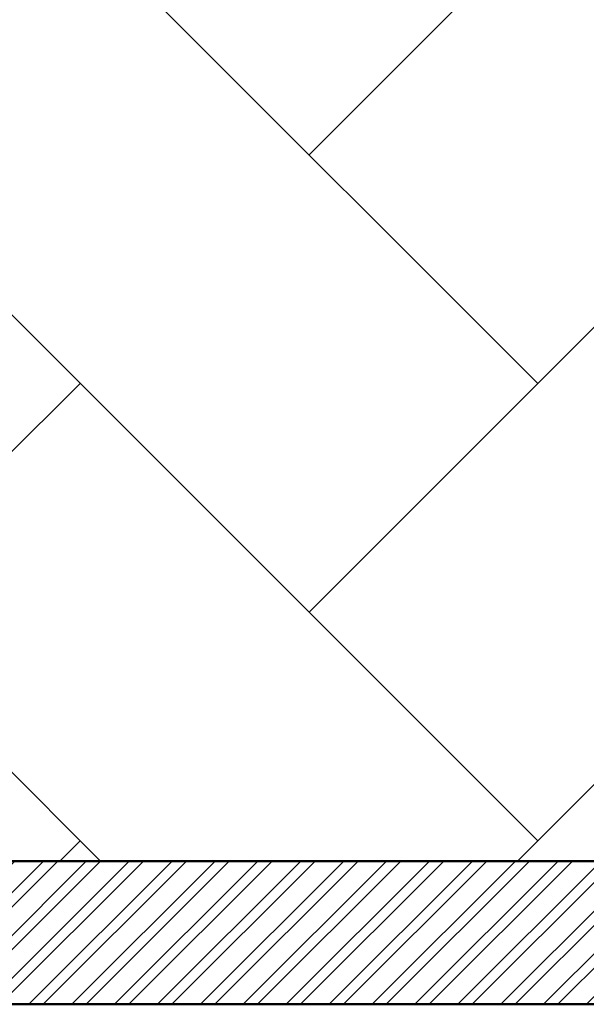
# Model space of a CAD drawing. Units: inches. Extents: x 3590 to 5167, y 65 to 1917.
# Tile 35 of 100: x 4968 to 5003, y 1326 to 1388. Entities that reach past the tile are written whole.
import ezdxf

# ---------------------------------------------------------------- set-up
doc = ezdxf.new("R2010")
doc.units = ezdxf.units.IN
for name, color, linetype, lineweight in [('A-FLOR-PATT', 8, 'Continuous', 13), ('A-WALL', 7, 'Continuous', 50), ('A-WALL-PATT', 251, 'Continuous', 13)]:
    doc.layers.add(name, color=color, linetype=linetype, lineweight=lineweight)

msp = doc.modelspace()

# ---------------------------------------------------------------- hatches: boundary and pattern name
at = {"layer": 'A-FLOR-PATT', "transparency": 33554687}
h = msp.add_hatch(dxfattribs=at)
h.set_pattern_fill('AR-HBONE', color=256, scale=0.2)
h.set_pattern_definition([(45, (-588.972, 0), (0, 28.73682), [60.96, -20.32]), (135, (-574.604, 14.368), (3e-15, 28.73682), [60.96, -20.32])])
h.paths.add_polyline_path([(5071.274, 1796.999), (4933.274, 1796.999), (4933.274, 1753.999), (4962.774, 1753.999, -0.414214), (4928.774, 1719.999), (4933.274, 1718.999), (4933.274, 1334.999), (5071.274, 1334.999)])
h.paths.add_polyline_path([(4951.78, 1521.077), (4951.715, 1521.04), (4951.563, 1520.895)], flags=16)
h.paths.add_polyline_path([(4952.267, 1521.376), (4952.198, 1521.371), (4952.198, 1521.356)], flags=0)
h.paths.add_polyline_path([(4967.051, 1529.728), (4965.231, 1528.694), (4963.411, 1527.714), (4961.756, 1526.851), (4963.589, 1527.449), (4964.036, 1527.478), (4962.975, 1527.249), (4961.76, 1526.852), (4959.792, 1525.834), (4958.005, 1524.895), (4956.24, 1523.93), (4954.504, 1522.919), (4954.129, 1522.682), (4953.361, 1521.997), (4953.366, 1521.998), (4953.605, 1522.064), (4955.106, 1522.761), (4956.921, 1523.434), (4958.678, 1523.915), (4960.358, 1524.2), (4961.945, 1524.286), (4964.171, 1524.108), (4965.958, 1523.309), (4963.863, 1522.976), (4965.187, 1522.499), (4963.366, 1522.497), (4961.545, 1522.487), (4959.764, 1522.461), (4958.304, 1522.419), (4957.974, 1522.388), (4956.307, 1522.232), (4954.718, 1522.071), (4953.251, 1521.899), (4953.525, 1521.623), (4954.331, 1521.379), (4956.243, 1521.23), (4958.039, 1520.93), (4959.684, 1520.483), (4961.16, 1519.896), (4963.107, 1518.8), (4964.393, 1517.325), (4962.973, 1517.726), (4964.558, 1516.661), (4965.407, 1515.708), (4963.507, 1516.322), (4961.68, 1517.005), (4959.935, 1517.745), (4958.282, 1518.528), (4956.732, 1519.343), (4955.295, 1520.175), (4954.672, 1520.572), (4954.513, 1520.627), (4955.658, 1519.318), (4956.703, 1517.982), (4957.644, 1516.647), (4958.485, 1515.334), (4959.55, 1513.524), (4960.438, 1511.769), (4958.841, 1513.62), (4957.452, 1515.325), (4955.819, 1517.459), (4956.665, 1515.448), (4957.111, 1513.923), (4957.447, 1511.714), (4957.076, 1509.793), (4956.538, 1511.11), (4955.992, 1512.569), (4955.444, 1514.125), (4954.898, 1515.735), (4954.357, 1517.356), (4953.824, 1518.943), (4953.305, 1520.452), (4953.065, 1521.116), (4952.971, 1521.146), (4952.949, 1521.086), (4952.73, 1520.199), (4953.37, 1518.024), (4953.757, 1516.373), (4954.051, 1514.765), (4954.264, 1513.221), (4954.471, 1511.131), (4954.497, 1510.402), (4954.409, 1511.76), (4954.264, 1513.221), (4954.051, 1514.765), (4953.757, 1516.373), (4953.37, 1518.024), (4952.877, 1519.698), (4952.716, 1520.141), (4952.533, 1519.059), (4952.374, 1517.789), (4952.219, 1516.312), (4952.046, 1514.6), (4951.833, 1512.626), (4951.557, 1510.363), (4951.203, 1512.168), (4950.852, 1514.339), (4950.985, 1516.376), (4951.66, 1518.286), (4952.593, 1520.481), (4952.357, 1521.13), (4951.855, 1520.328), (4950.839, 1518.908), (4949.777, 1517.587), (4948.916, 1516.617), (4948.111, 1515.256), (4947.089, 1513.554), (4945.889, 1511.615), (4946.326, 1513.402), (4946.562, 1514.249), (4945.528, 1513.327), (4944.581, 1512.531), (4946.018, 1514.508), (4947.204, 1516.048), (4947.893, 1517.313), (4949.307, 1518.764), (4950.414, 1519.767), (4950.451, 1519.806), (4952.267, 1521.376), (4951.645, 1521.493), (4950.404, 1521.18), (4948.044, 1520.359), (4946.119, 1519.452), (4944.572, 1518.475), (4943.35, 1517.443), (4941.997, 1515.92), (4941.661, 1515.275), (4942.813, 1516.99), (4944.572, 1518.475), (4946.119, 1519.452), (4948.044, 1520.359), (4950.404, 1521.18), (4951.645, 1521.493), (4949.647, 1521.868), (4948.6, 1521.756), (4947.126, 1521.57), (4945.42, 1521.348), (4943.45, 1521.105), (4941.183, 1520.856), (4942.86, 1521.613), (4943.873, 1522.03), (4942.952, 1521.909), (4941.41, 1521.485), (4939.543, 1520.67), (4938.968, 1520.226), (4940.733, 1521.299), (4942.952, 1521.909), (4943.702, 1522.008), (4945.894, 1522.7), (4947.565, 1522.714), (4948.921, 1522.566), (4951.131, 1522.183), (4950.971, 1522.297), (4948.129, 1523.006), (4946.035, 1523.707), (4944.232, 1524.521), (4942.707, 1525.461), (4941.444, 1526.537), (4940.43, 1527.761), (4939.649, 1529.143), (4941.421, 1528.122), (4943.147, 1527.132), (4944.841, 1526.175), (4946.514, 1525.25), (4948.179, 1524.359), (4948.365, 1524.263), (4946.475, 1526.045), (4945.181, 1527.54), (4944.19, 1529.033), (4943.496, 1530.54), (4943.278, 1531.36), (4942.498, 1531.919), (4943.114, 1531.762), (4942.959, 1533.659), (4944.14, 1531.989), (4944.612, 1531.323), (4946.202, 1530.463), (4947.486, 1529.509), (4948.79, 1528.226), (4950.368, 1526.237), (4949.485, 1528.155), (4948.851, 1530.123), (4948.491, 1532.041), (4948.381, 1533.918), (4948.501, 1535.76), (4948.827, 1537.573), (4949.418, 1535.565), (4949.957, 1533.569), (4950.464, 1531.586), (4950.961, 1529.617), (4951.391, 1527.954), (4951.724, 1530.687), (4952.201, 1532.58), (4952.889, 1534.33), (4953.77, 1535.951), (4954.827, 1537.46), (4954.521, 1535.39), (4954.273, 1533.937), (4955.58, 1535.663), (4956.748, 1536.739), (4956.159, 1534.78), (4955.589, 1532.873), (4955.043, 1531.006), (4954.525, 1529.166), (4954.038, 1527.341), (4953.638, 1525.733), (4953.611, 1525.586), (4953.398, 1524.166), (4953.382, 1524.009), (4954.07, 1525.476), (4954.912, 1527.022), (4956.136, 1528.894), (4957.847, 1530.577), (4959.376, 1531.54), (4958.256, 1530.104), (4957.143, 1528.663), (4956.066, 1527.243), (4955.056, 1525.871), (4954.141, 1524.571), (4953.352, 1523.372), (4953.311, 1523.303), (4953.273, 1522.925), (4953.261, 1522.382), (4954.103, 1523.373), (4954.63, 1524.284), (4955.961, 1526.358), (4957.23, 1528.13), (4958.421, 1529.609), (4960.037, 1531.368), (4961.374, 1532.375), (4962.101, 1532.77), (4961.07, 1531.061), (4959.987, 1529.438), (4958.869, 1527.908), (4958.15, 1527.007), (4959.803, 1528.003), (4961.589, 1528.793), (4963.391, 1529.328), (4965.211, 1529.632)], flags=16)
h.paths.add_polyline_path([(4962.944, 1523.182), (4961.107, 1523.422), (4960.392, 1523.362), (4962.35, 1523.331)], flags=0)
h.paths.add_polyline_path([(5049.541, 1584.551), (5049.476, 1584.515), (5049.325, 1584.37)], flags=16)
h.paths.add_polyline_path([(5050.028, 1584.851), (5049.959, 1584.845), (5049.959, 1584.83)], flags=0)
h.paths.add_polyline_path([(5042.333, 1581.949), (5043.88, 1582.926), (5045.806, 1583.833), (5048.165, 1584.654), (5049.406, 1584.967), (5047.408, 1585.342), (5046.361, 1585.231), (5044.888, 1585.044), (5043.181, 1584.822), (5041.211, 1584.579), (5038.944, 1584.33), (5040.622, 1585.087), (5041.634, 1585.504), (5040.713, 1585.383), (5039.171, 1584.959), (5037.304, 1584.144), (5036.729, 1583.7), (5038.494, 1584.773), (5040.713, 1585.383), (5041.463, 1585.482), (5043.655, 1586.174), (5045.326, 1586.188), (5046.682, 1586.04), (5048.893, 1585.657), (5048.732, 1585.771), (5045.891, 1586.48), (5043.796, 1587.181), (5041.994, 1587.996), (5040.468, 1588.935), (5039.205, 1590.011), (5038.191, 1591.235), (5037.41, 1592.617), (5039.182, 1591.596), (5040.909, 1590.607), (5042.602, 1589.649), (5044.275, 1588.724), (5045.94, 1587.833), (5046.126, 1587.738), (5044.237, 1589.519), (5042.942, 1591.015), (5041.952, 1592.508), (5041.257, 1594.014), (5041.039, 1594.834), (5040.26, 1595.393), (5040.875, 1595.237), (5040.721, 1597.133), (5041.901, 1595.463), (5042.373, 1594.798), (5043.963, 1593.938), (5045.247, 1592.983), (5046.552, 1591.701), (5048.129, 1589.712), (5047.247, 1591.63), (5046.613, 1593.597), (5046.252, 1595.515), (5046.142, 1597.392), (5046.262, 1599.234), (5046.588, 1601.047), (5047.179, 1599.039), (5047.718, 1597.043), (5048.225, 1595.06), (5048.722, 1593.091), (5049.152, 1591.429), (5049.485, 1594.161), (5049.962, 1596.054), (5050.65, 1597.804), (5051.532, 1599.425), (5052.589, 1600.934), (5052.283, 1598.864), (5052.034, 1597.411), (5053.341, 1599.137), (5054.509, 1600.213), (5053.92, 1598.254), (5053.35, 1596.348), (5052.805, 1594.48), (5052.286, 1592.64), (5051.799, 1590.815), (5051.4, 1589.207), (5051.373, 1589.06), (5051.159, 1587.64), (5051.143, 1587.483), (5051.831, 1588.95), (5052.673, 1590.496), (5053.898, 1592.368), (5055.608, 1594.051), (5057.137, 1595.014), (5056.017, 1593.578), (5054.904, 1592.137), (5053.828, 1590.717), (5052.817, 1589.345), (5051.902, 1588.046), (5051.113, 1586.846), (5051.072, 1586.777), (5051.034, 1586.399), (5051.022, 1585.856), (5051.864, 1586.847), (5052.391, 1587.758), (5053.723, 1589.832), (5054.991, 1591.604), (5056.182, 1593.083), (5057.798, 1594.842), (5059.135, 1595.849), (5059.863, 1596.244), (5058.831, 1594.535), (5057.749, 1592.912), (5056.63, 1591.382), (5055.912, 1590.482), (5057.564, 1591.477), (5059.35, 1592.267), (5061.152, 1592.802), (5062.972, 1593.106), (5064.812, 1593.203), (5062.992, 1592.169), (5061.172, 1591.188), (5059.518, 1590.325), (5061.35, 1590.924), (5061.797, 1590.952), (5060.737, 1590.723), (5059.521, 1590.326), (5057.553, 1589.308), (5055.766, 1588.369), (5054.002, 1587.404), (5052.265, 1586.393), (5051.891, 1586.156), (5051.122, 1585.471), (5051.127, 1585.472), (5051.366, 1585.538), (5052.867, 1586.235), (5054.682, 1586.908), (5056.439, 1587.389), (5058.12, 1587.675), (5059.706, 1587.76), (5061.933, 1587.583), (5063.719, 1586.783), (5061.624, 1586.45), (5062.949, 1585.973), (5061.127, 1585.971), (5059.307, 1585.961), (5057.525, 1585.935), (5056.065, 1585.893), (5055.735, 1585.862), (5054.068, 1585.707), (5052.479, 1585.546), (5051.012, 1585.373), (5051.286, 1585.097), (5052.092, 1584.853), (5054.004, 1584.704), (5055.8, 1584.404), (5057.446, 1583.958), (5058.921, 1583.37), (5060.868, 1582.274), (5062.154, 1580.799), (5060.734, 1581.2), (5062.32, 1580.135), (5063.168, 1579.182), (5061.269, 1579.796), (5059.441, 1580.479), (5057.696, 1581.219), (5056.043, 1582.003), (5054.493, 1582.817), (5053.057, 1583.649), (5052.433, 1584.047), (5052.274, 1584.101), (5053.42, 1582.793), (5054.464, 1581.457), (5055.405, 1580.121), (5056.247, 1578.809), (5057.311, 1576.998), (5058.199, 1575.244), (5056.602, 1577.094), (5055.213, 1578.799), (5053.58, 1580.933), (5054.427, 1578.922), (5054.872, 1577.397), (5055.208, 1575.189), (5054.838, 1573.267), (5054.299, 1574.584), (5053.754, 1576.043), (5053.206, 1577.599), (5052.659, 1579.209), (5052.118, 1580.83), (5051.585, 1582.417), (5051.066, 1583.927), (5050.826, 1584.59), (5050.733, 1584.62), (5050.711, 1584.561), (5050.491, 1583.673), (5051.131, 1581.498), (5051.518, 1579.847), (5051.813, 1578.24), (5052.026, 1576.695), (5052.233, 1574.605), (5052.258, 1573.876), (5052.17, 1575.234), (5052.026, 1576.695), (5051.813, 1578.24), (5051.518, 1579.847), (5051.131, 1581.498), (5050.638, 1583.172), (5050.477, 1583.615), (5050.294, 1582.533), (5050.136, 1581.263), (5049.981, 1579.786), (5049.807, 1578.074), (5049.594, 1576.1), (5049.318, 1573.837), (5048.965, 1575.642), (5048.613, 1577.813), (5048.747, 1579.85), (5049.421, 1581.76), (5050.354, 1583.955), (5050.118, 1584.604), (5049.616, 1583.802), (5048.6, 1582.382), (5047.538, 1581.061), (5046.677, 1580.091), (5045.872, 1578.73), (5044.85, 1577.028), (5043.651, 1575.089), (5044.087, 1576.877), (5044.324, 1577.723), (5043.289, 1576.801), (5042.342, 1576.005), (5043.779, 1577.982), (5044.966, 1579.522), (5045.655, 1580.787), (5047.068, 1582.239), (5048.175, 1583.241), (5048.213, 1583.28), (5050.028, 1584.851), (5049.406, 1584.967), (5048.165, 1584.654), (5045.806, 1583.833), (5043.88, 1582.926), (5042.333, 1581.949), (5041.111, 1580.917), (5039.758, 1579.394), (5039.423, 1578.749), (5040.575, 1580.464)], flags=16)
h.paths.add_polyline_path([(4954.799, 1533.12), (4954.262, 1532.079), (4953.831, 1530.935), (4953.505, 1529.636), (4953.283, 1528.133), (4953.167, 1526.376), (4953.156, 1524.315), (4953.277, 1521.236), (4952.802, 1521.842), (4951.557, 1521.998), (4950.976, 1521.961), (4952.661, 1521.941), (4952.802, 1521.842), (4953.152, 1523.593), (4953.167, 1526.376), (4953.283, 1528.133), (4953.609, 1530.346), (4954.456, 1532.592)], flags=0)
h.paths.add_polyline_path([(5050.563, 1585.316), (5049.318, 1585.472), (5048.737, 1585.435), (5050.422, 1585.415), (5050.563, 1585.316), (5050.914, 1587.067), (5050.928, 1589.851), (5051.045, 1591.607), (5051.371, 1593.82), (5052.217, 1596.066), (5052.56, 1596.594), (5052.024, 1595.554), (5051.592, 1594.409), (5051.266, 1593.11), (5051.045, 1591.607), (5050.928, 1589.851), (5050.918, 1587.789), (5051.038, 1584.71)], flags=0)
h.paths.add_polyline_path([(5058.153, 1586.836), (5060.111, 1586.805), (5060.705, 1586.656), (5058.868, 1586.896)], flags=0)
h.paths.add_polyline_path([(5049.541, 1430.936), (5049.476, 1430.9), (5049.325, 1430.755)], flags=16)
h.paths.add_polyline_path([(5050.028, 1431.236), (5049.959, 1431.231), (5049.959, 1431.215)], flags=0)
h.paths.add_polyline_path([(5046.588, 1447.432), (5047.179, 1445.425), (5047.718, 1443.429), (5048.225, 1441.446), (5048.722, 1439.476), (5049.152, 1437.814), (5049.485, 1440.546), (5049.962, 1442.439), (5050.65, 1444.189), (5051.532, 1445.811), (5052.589, 1447.319), (5052.283, 1445.249), (5052.034, 1443.796), (5053.341, 1445.522), (5054.509, 1446.598), (5053.92, 1444.64), (5053.35, 1442.733), (5052.805, 1440.865), (5052.286, 1439.025), (5051.799, 1437.201), (5051.4, 1435.592), (5051.373, 1435.445), (5051.159, 1434.025), (5051.143, 1433.868), (5051.831, 1435.335), (5052.673, 1436.881), (5053.898, 1438.753), (5055.608, 1440.436), (5057.137, 1441.4), (5056.017, 1439.963), (5054.904, 1438.522), (5053.828, 1437.102), (5052.817, 1435.73), (5051.902, 1434.431), (5051.113, 1433.231), (5051.072, 1433.162), (5051.034, 1432.784), (5051.022, 1432.242), (5051.864, 1433.232), (5052.391, 1434.143), (5053.723, 1436.217), (5054.991, 1437.989), (5056.182, 1439.468), (5057.798, 1441.227), (5059.135, 1442.235), (5059.863, 1442.629), (5058.831, 1440.921), (5057.749, 1439.298), (5056.63, 1437.767), (5055.912, 1436.867), (5057.564, 1437.863), (5059.35, 1438.652), (5061.152, 1439.187), (5062.972, 1439.491), (5064.812, 1439.588), (5062.992, 1438.554), (5061.172, 1437.573), (5059.518, 1436.71), (5061.35, 1437.309), (5061.797, 1437.337), (5060.737, 1437.108), (5059.521, 1436.711), (5057.553, 1435.693), (5055.766, 1434.754), (5054.002, 1433.789), (5052.265, 1432.778), (5051.891, 1432.541), (5051.122, 1431.856), (5051.127, 1431.857), (5051.366, 1431.923), (5052.867, 1432.62), (5054.682, 1433.293), (5056.439, 1433.775), (5058.12, 1434.06), (5059.706, 1434.145), (5061.933, 1433.968), (5063.719, 1433.168), (5061.624, 1432.835), (5062.949, 1432.358), (5061.127, 1432.357), (5059.307, 1432.346), (5057.525, 1432.32), (5056.065, 1432.278), (5055.735, 1432.248), (5054.068, 1432.092), (5052.479, 1431.931), (5051.012, 1431.759), (5051.286, 1431.482), (5052.092, 1431.238), (5054.004, 1431.089), (5055.8, 1430.789), (5057.446, 1430.343), (5058.921, 1429.755), (5060.868, 1428.66), (5062.154, 1427.185), (5060.734, 1427.585), (5062.32, 1426.52), (5063.168, 1425.567), (5061.269, 1426.181), (5059.441, 1426.865), (5057.696, 1427.604), (5056.043, 1428.388), (5054.493, 1429.202), (5053.057, 1430.034), (5052.433, 1430.432), (5052.274, 1430.487), (5053.42, 1429.178), (5054.464, 1427.842), (5055.405, 1426.506), (5056.247, 1425.194), (5057.311, 1423.383), (5058.199, 1421.629), (5056.602, 1423.479), (5055.213, 1425.184), (5053.58, 1427.318), (5054.427, 1425.307), (5054.872, 1423.782), (5055.208, 1421.574), (5054.838, 1419.652), (5054.299, 1420.97), (5053.754, 1422.428), (5053.206, 1423.984), (5052.659, 1425.595), (5052.118, 1427.215), (5051.585, 1428.802), (5051.066, 1430.312), (5050.826, 1430.975), (5050.733, 1431.005), (5050.711, 1430.946), (5050.491, 1430.058), (5051.131, 1427.883), (5051.518, 1426.232), (5051.813, 1424.625), (5052.026, 1423.081), (5052.233, 1420.991), (5052.258, 1420.261), (5052.17, 1421.619), (5052.026, 1423.081), (5051.813, 1424.625), (5051.518, 1426.232), (5051.131, 1427.883), (5050.638, 1429.558), (5050.477, 1430.001), (5050.294, 1428.918), (5050.136, 1427.648), (5049.981, 1426.171), (5049.807, 1424.459), (5049.594, 1422.485), (5049.318, 1420.222), (5048.965, 1422.028), (5048.613, 1424.199), (5048.747, 1426.235), (5049.421, 1428.146), (5050.354, 1430.34), (5050.118, 1430.989), (5049.616, 1430.187), (5048.6, 1428.768), (5047.538, 1427.446), (5046.677, 1426.477), (5045.872, 1425.116), (5044.85, 1423.413), (5043.651, 1421.474), (5044.087, 1423.262), (5044.324, 1424.109), (5043.289, 1423.186), (5042.342, 1422.391), (5043.779, 1424.368), (5044.966, 1425.907), (5045.655, 1427.173), (5047.068, 1428.624), (5048.175, 1429.627), (5048.213, 1429.666), (5050.028, 1431.236), (5049.406, 1431.353), (5048.165, 1431.039), (5045.806, 1430.218), (5043.88, 1429.311), (5042.333, 1428.334), (5041.111, 1427.302), (5039.758, 1425.779), (5039.423, 1425.134), (5040.575, 1426.849), (5042.333, 1428.334), (5043.88, 1429.311), (5045.806, 1430.218), (5048.165, 1431.039), (5049.406, 1431.353), (5047.408, 1431.727), (5046.361, 1431.616), (5044.888, 1431.429), (5043.181, 1431.207), (5041.211, 1430.964), (5038.944, 1430.715), (5040.622, 1431.472), (5041.634, 1431.89), (5040.713, 1431.769), (5039.171, 1431.345), (5037.304, 1430.53), (5036.729, 1430.085), (5038.494, 1431.158), (5040.713, 1431.769), (5041.463, 1431.867), (5043.655, 1432.559), (5045.326, 1432.573), (5046.682, 1432.425), (5048.893, 1432.042), (5048.732, 1432.156), (5045.891, 1432.865), (5043.796, 1433.566), (5041.994, 1434.381), (5040.468, 1435.321), (5039.205, 1436.396), (5038.191, 1437.62), (5037.41, 1439.002), (5039.182, 1437.982), (5040.909, 1436.992), (5042.602, 1436.034), (5044.275, 1435.109), (5045.94, 1434.218), (5046.126, 1434.123), (5044.237, 1435.904), (5042.942, 1437.4), (5041.952, 1438.893), (5041.257, 1440.399), (5041.039, 1441.219), (5040.26, 1441.778), (5040.875, 1441.622), (5040.721, 1443.518), (5041.901, 1441.848), (5042.373, 1441.183), (5043.963, 1440.323), (5045.247, 1439.369), (5046.552, 1438.086), (5048.129, 1436.097), (5047.247, 1438.015), (5046.613, 1439.982), (5046.252, 1441.901), (5046.142, 1443.778), (5046.262, 1445.619)], flags=16)
h.paths.add_polyline_path([(5052.382, 1444.255), (5051.623, 1442.78), (5052.024, 1441.939), (5052.56, 1442.98)], flags=0)
h.paths.add_polyline_path([(5050.563, 1431.701), (5049.318, 1431.857), (5048.737, 1431.821), (5050.422, 1431.8)], flags=0)
h.paths.add_polyline_path([(5058.153, 1433.221), (5060.111, 1433.19), (5060.705, 1433.041), (5058.868, 1433.281)], flags=0)
h.paths.add_polyline_path([(5049.541, 1352.285), (5049.476, 1352.249), (5049.325, 1352.104)], flags=16)
h.paths.add_polyline_path([(5050.028, 1352.585), (5049.959, 1352.58), (5049.959, 1352.564)], flags=0)
h.paths.add_polyline_path([(5046.588, 1368.781), (5047.179, 1366.774), (5047.718, 1364.778), (5048.225, 1362.795), (5048.722, 1360.825), (5049.152, 1359.163), (5049.485, 1361.896), (5049.962, 1363.789), (5050.65, 1365.538), (5051.532, 1367.16), (5052.589, 1368.669), (5052.283, 1366.598), (5052.034, 1365.145), (5053.341, 1366.871), (5054.509, 1367.947), (5053.92, 1365.989), (5053.35, 1364.082), (5052.805, 1362.214), (5052.286, 1360.374), (5051.799, 1358.55), (5051.4, 1356.942), (5051.373, 1356.794), (5051.159, 1355.374), (5051.143, 1355.218), (5051.831, 1356.684), (5052.673, 1358.23), (5053.898, 1360.102), (5055.608, 1361.786), (5057.137, 1362.749), (5056.017, 1361.313), (5054.904, 1359.872), (5053.828, 1358.452), (5052.817, 1357.079), (5051.902, 1355.78), (5051.113, 1354.581), (5051.072, 1354.512), (5051.034, 1354.133), (5051.022, 1353.591), (5051.864, 1354.581), (5052.391, 1355.492), (5053.723, 1357.566), (5054.991, 1359.338), (5056.182, 1360.817), (5057.798, 1362.577), (5059.135, 1363.584), (5059.863, 1363.979), (5058.831, 1362.27), (5057.749, 1360.647), (5056.63, 1359.117), (5055.912, 1358.216), (5057.564, 1359.212), (5059.35, 1360.001), (5061.152, 1360.536), (5062.972, 1360.841), (5064.812, 1360.937), (5062.992, 1359.903), (5061.172, 1358.923), (5059.518, 1358.059), (5061.35, 1358.658), (5061.797, 1358.687), (5060.737, 1358.458), (5059.521, 1358.061), (5057.553, 1357.043), (5055.766, 1356.103), (5054.002, 1355.138), (5052.265, 1354.127), (5051.891, 1353.89), (5051.122, 1353.206), (5051.127, 1353.206), (5051.366, 1353.272), (5052.867, 1353.969), (5054.682, 1354.643), (5056.439, 1355.124), (5058.12, 1355.409), (5059.706, 1355.495), (5061.933, 1355.317), (5063.719, 1354.518), (5061.624, 1354.184), (5062.949, 1353.708), (5061.127, 1353.706), (5059.307, 1353.695), (5057.525, 1353.669), (5056.065, 1353.627), (5055.735, 1353.597), (5054.068, 1353.441), (5052.479, 1353.28), (5051.012, 1353.108), (5051.286, 1352.831), (5052.092, 1352.587), (5054.004, 1352.439), (5055.8, 1352.138), (5057.446, 1351.692), (5058.921, 1351.104), (5060.868, 1350.009), (5062.154, 1348.534), (5060.734, 1348.935), (5062.32, 1347.869), (5063.168, 1346.916), (5061.269, 1347.53), (5059.441, 1348.214), (5057.696, 1348.954), (5056.043, 1349.737), (5054.493, 1350.551), (5053.057, 1351.383), (5052.433, 1351.781), (5052.274, 1351.836), (5053.42, 1350.527), (5054.464, 1349.191), (5055.405, 1347.855), (5056.247, 1346.543), (5057.311, 1344.733), (5058.199, 1342.978), (5056.602, 1344.828), (5055.213, 1346.534), (5053.58, 1348.667), (5054.427, 1346.656), (5054.872, 1345.132), (5055.208, 1342.923), (5054.838, 1341.002), (5054.299, 1342.319), (5053.754, 1343.778), (5053.206, 1345.334), (5052.659, 1346.944), (5052.118, 1348.564), (5051.585, 1350.151), (5051.066, 1351.661), (5050.826, 1352.324), (5050.733, 1352.355), (5050.711, 1352.295), (5050.491, 1351.408), (5051.131, 1349.232), (5051.518, 1347.581), (5051.813, 1345.974), (5052.026, 1344.43), (5052.233, 1342.34), (5052.258, 1341.61), (5052.17, 1342.969), (5052.026, 1344.43), (5051.813, 1345.974), (5051.518, 1347.581), (5051.131, 1349.232), (5050.638, 1350.907), (5050.477, 1351.35), (5050.294, 1350.267), (5050.136, 1348.997), (5049.981, 1347.52), (5049.807, 1345.809), (5049.594, 1343.835), (5049.318, 1341.571), (5048.965, 1343.377), (5048.613, 1345.548), (5048.747, 1347.585), (5049.421, 1349.495), (5050.354, 1351.689), (5050.118, 1352.339), (5049.616, 1351.536), (5048.6, 1350.117), (5047.538, 1348.795), (5046.677, 1347.826), (5045.872, 1346.465), (5044.85, 1344.763), (5043.651, 1342.824), (5044.087, 1344.611), (5044.324, 1345.458), (5043.289, 1344.535), (5042.342, 1343.74), (5043.779, 1345.717), (5044.966, 1347.256), (5045.655, 1348.522), (5047.068, 1349.973), (5048.175, 1350.976), (5048.213, 1351.015), (5050.028, 1352.585), (5049.406, 1352.702), (5048.165, 1352.388), (5045.806, 1351.567), (5043.88, 1350.661), (5042.333, 1349.683), (5041.111, 1348.651), (5039.758, 1347.128), (5039.423, 1346.483), (5040.575, 1348.198), (5042.333, 1349.683), (5043.88, 1350.661), (5045.806, 1351.567), (5048.165, 1352.388), (5049.406, 1352.702), (5047.408, 1353.076), (5046.361, 1352.965), (5044.888, 1352.779), (5043.181, 1352.556), (5041.211, 1352.313), (5038.944, 1352.065), (5040.622, 1352.821), (5041.634, 1353.239), (5040.713, 1353.118), (5039.171, 1352.694), (5037.304, 1351.879), (5036.729, 1351.434), (5038.494, 1352.508), (5040.713, 1353.118), (5041.463, 1353.216), (5043.655, 1353.909), (5045.326, 1353.923), (5046.682, 1353.774), (5048.893, 1353.391), (5048.732, 1353.506), (5045.891, 1354.214), (5043.796, 1354.915), (5041.994, 1355.73), (5040.468, 1356.67), (5039.205, 1357.746), (5038.191, 1358.969), (5037.41, 1360.352), (5039.182, 1359.331), (5040.909, 1358.341), (5042.602, 1357.383), (5044.275, 1356.458), (5045.94, 1355.567), (5046.126, 1355.472), (5044.237, 1357.253), (5042.942, 1358.749), (5041.952, 1360.242), (5041.257, 1361.748), (5041.039, 1362.568), (5040.26, 1363.128), (5040.875, 1362.971), (5040.721, 1364.867), (5041.901, 1363.197), (5042.373, 1362.532), (5043.963, 1361.672), (5045.247, 1360.718), (5046.552, 1359.435), (5048.129, 1357.446), (5047.247, 1359.364), (5046.613, 1361.331), (5046.252, 1363.25), (5046.142, 1365.127), (5046.262, 1366.969)], flags=16)
h.paths.add_polyline_path([(5052.382, 1365.604), (5051.623, 1364.129), (5052.024, 1363.288), (5052.56, 1364.329)], flags=0)
h.paths.add_polyline_path([(4951.78, 1698.041), (4951.715, 1698.005), (4951.563, 1697.859)], flags=16)
h.paths.add_polyline_path([(4952.267, 1698.341), (4952.198, 1698.335), (4952.198, 1698.32)], flags=0)
h.paths.add_polyline_path([(4957.076, 1686.757), (4956.538, 1688.074), (4955.992, 1689.533), (4955.444, 1691.089), (4954.898, 1692.699), (4954.357, 1694.32), (4953.824, 1695.907), (4953.305, 1697.417), (4953.065, 1698.08), (4952.971, 1698.11), (4952.949, 1698.051), (4952.73, 1697.163), (4953.37, 1694.988), (4953.757, 1693.337), (4954.051, 1691.729), (4954.264, 1690.185), (4954.471, 1688.095), (4954.497, 1687.366), (4954.409, 1688.724), (4954.264, 1690.185), (4954.051, 1691.729), (4953.757, 1693.337), (4953.37, 1694.988), (4952.877, 1696.662), (4952.716, 1697.105), (4952.533, 1696.023), (4952.374, 1694.753), (4952.219, 1693.276), (4952.046, 1691.564), (4951.833, 1689.59), (4951.557, 1687.327), (4951.203, 1689.132), (4950.852, 1691.303), (4950.985, 1693.34), (4951.66, 1695.25), (4952.593, 1697.445), (4952.357, 1698.094), (4951.855, 1697.292), (4950.839, 1695.872), (4949.777, 1694.551), (4948.916, 1693.581), (4948.111, 1692.22), (4947.089, 1690.518), (4945.889, 1688.579), (4946.326, 1690.366), (4946.562, 1691.213), (4945.528, 1690.291), (4944.581, 1689.495), (4946.018, 1691.472), (4947.204, 1693.012), (4947.893, 1694.277), (4949.307, 1695.729), (4950.414, 1696.731), (4950.451, 1696.77), (4952.267, 1698.341), (4951.645, 1698.457), (4950.404, 1698.144), (4948.044, 1697.323), (4946.119, 1696.416), (4944.572, 1695.439), (4943.35, 1694.407), (4941.997, 1692.884), (4941.661, 1692.239), (4942.813, 1693.954), (4944.572, 1695.439), (4946.119, 1696.416), (4948.044, 1697.323), (4950.404, 1698.144), (4951.645, 1698.457), (4949.647, 1698.832), (4948.6, 1698.72), (4947.126, 1698.534), (4945.42, 1698.312), (4943.45, 1698.069), (4941.183, 1697.82), (4942.86, 1698.577), (4943.873, 1698.994), (4942.952, 1698.873), (4941.41, 1698.449), (4939.543, 1697.634), (4938.968, 1697.19), (4940.733, 1698.263), (4942.952, 1698.873), (4943.702, 1698.972), (4945.894, 1699.664), (4947.565, 1699.678), (4948.921, 1699.53), (4951.131, 1699.147), (4950.971, 1699.261), (4948.129, 1699.97), (4946.035, 1700.671), (4944.232, 1701.486), (4942.707, 1702.425), (4941.444, 1703.501), (4940.43, 1704.725), (4939.649, 1706.107), (4941.421, 1705.086), (4943.147, 1704.097), (4944.841, 1703.139), (4946.514, 1702.214), (4948.179, 1701.323), (4948.365, 1701.227), (4946.475, 1703.009), (4945.181, 1704.505), (4944.19, 1705.997), (4943.496, 1707.504), (4943.278, 1708.324), (4942.498, 1708.883), (4943.114, 1708.727), (4942.959, 1710.623), (4944.14, 1708.953), (4944.612, 1708.287), (4946.202, 1707.428), (4947.486, 1706.473), (4948.79, 1705.191), (4950.368, 1703.202), (4949.485, 1705.12), (4948.851, 1707.087), (4948.491, 1709.005), (4948.381, 1710.882), (4948.501, 1712.724), (4948.827, 1714.537), (4949.418, 1712.529), (4949.957, 1710.533), (4950.464, 1708.55), (4950.961, 1706.581), (4951.391, 1704.919), (4951.724, 1707.651), (4952.201, 1709.544), (4952.889, 1711.294), (4953.77, 1712.915), (4954.827, 1714.424), (4954.521, 1712.354), (4954.273, 1710.901), (4955.58, 1712.627), (4956.748, 1713.703), (4956.159, 1711.744), (4955.589, 1709.837), (4955.043, 1707.97), (4954.525, 1706.13), (4954.038, 1704.305), (4953.638, 1702.697), (4953.611, 1702.55), (4953.398, 1701.13), (4953.382, 1700.973), (4954.07, 1702.44), (4954.912, 1703.986), (4956.136, 1705.858), (4957.847, 1707.541), (4959.376, 1708.504), (4958.256, 1707.068), (4957.143, 1705.627), (4956.066, 1704.207), (4955.056, 1702.835), (4954.141, 1701.536), (4953.352, 1700.336), (4953.311, 1700.267), (4953.273, 1699.889), (4953.261, 1699.346), (4954.103, 1700.337), (4954.63, 1701.248), (4955.961, 1703.322), (4957.23, 1705.094), (4958.421, 1706.573), (4960.037, 1708.332), (4961.374, 1709.339), (4962.101, 1709.734), (4961.07, 1708.025), (4959.987, 1706.402), (4958.869, 1704.872), (4958.15, 1703.972), (4959.803, 1704.967), (4961.589, 1705.757), (4963.391, 1706.292), (4965.211, 1706.596), (4967.051, 1706.692), (4965.231, 1705.659), (4963.411, 1704.678), (4961.756, 1703.815), (4963.589, 1704.413), (4964.036, 1704.442), (4962.975, 1704.213), (4961.76, 1703.816), (4959.792, 1702.798), (4958.005, 1701.859), (4956.24, 1700.894), (4954.504, 1699.883), (4954.129, 1699.646), (4953.361, 1698.961), (4953.366, 1698.962), (4953.605, 1699.028), (4955.106, 1699.725), (4956.921, 1700.398), (4958.678, 1700.879), (4960.358, 1701.164), (4961.945, 1701.25), (4964.171, 1701.073), (4965.958, 1700.273), (4963.863, 1699.94), (4965.187, 1699.463), (4963.366, 1699.461), (4961.545, 1699.451), (4959.764, 1699.425), (4958.304, 1699.383), (4957.974, 1699.352), (4956.307, 1699.197), (4954.718, 1699.036), (4953.251, 1698.863), (4953.525, 1698.587), (4954.331, 1698.343), (4956.243, 1698.194), (4958.039, 1697.894), (4959.684, 1697.447), (4961.16, 1696.86), (4963.107, 1695.764), (4964.393, 1694.289), (4962.973, 1694.69), (4964.558, 1693.625), (4965.407, 1692.672), (4963.507, 1693.286), (4961.68, 1693.969), (4959.935, 1694.709), (4958.282, 1695.492), (4956.732, 1696.307), (4955.295, 1697.139), (4954.672, 1697.536), (4954.513, 1697.591), (4955.658, 1696.282), (4956.703, 1694.946), (4957.644, 1693.611), (4958.485, 1692.298), (4959.55, 1690.488), (4960.438, 1688.733), (4958.841, 1690.584), (4957.452, 1692.289), (4955.819, 1694.423), (4956.665, 1692.412), (4957.111, 1690.887), (4957.447, 1688.678)], flags=16)
h.paths.add_polyline_path([(5050.563, 1353.05), (5049.318, 1353.207), (5048.737, 1353.17), (5050.422, 1353.15)], flags=0)
h.paths.add_polyline_path([(4951.78, 1351.486), (4951.715, 1351.45), (4951.563, 1351.305)], flags=16)
h.paths.add_polyline_path([(4952.267, 1351.786), (4952.198, 1351.78), (4952.198, 1351.765)], flags=0)
h.paths.add_polyline_path([(4954.827, 1367.869), (4954.521, 1365.799), (4954.273, 1364.346), (4955.58, 1366.072), (4956.748, 1367.148), (4956.159, 1365.19), (4955.589, 1363.283), (4955.043, 1361.415), (4954.525, 1359.575), (4954.038, 1357.751), (4953.638, 1356.142), (4953.611, 1355.995), (4953.398, 1354.575), (4953.382, 1354.418), (4954.07, 1355.885), (4954.912, 1357.431), (4956.136, 1359.303), (4957.847, 1360.986), (4959.376, 1361.95), (4958.256, 1360.513), (4957.143, 1359.072), (4956.066, 1357.652), (4955.056, 1356.28), (4954.141, 1354.981), (4953.352, 1353.781), (4953.311, 1353.712), (4953.273, 1353.334), (4953.261, 1352.792), (4954.103, 1353.782), (4954.63, 1354.693), (4955.961, 1356.767), (4957.23, 1358.539), (4958.421, 1360.018), (4960.037, 1361.777), (4961.374, 1362.785), (4962.101, 1363.179), (4961.07, 1361.471), (4959.987, 1359.848), (4958.869, 1358.317), (4958.15, 1357.417), (4959.803, 1358.413), (4961.589, 1359.202), (4963.391, 1359.737), (4965.211, 1360.041), (4967.051, 1360.138), (4965.231, 1359.104), (4963.411, 1358.123), (4961.756, 1357.26), (4963.589, 1357.859), (4964.036, 1357.887), (4962.975, 1357.658), (4961.76, 1357.261), (4959.792, 1356.243), (4958.005, 1355.304), (4956.24, 1354.339), (4954.504, 1353.328), (4954.129, 1353.091), (4953.361, 1352.406), (4953.366, 1352.407), (4953.605, 1352.473), (4955.106, 1353.17), (4956.921, 1353.843), (4958.678, 1354.325), (4960.358, 1354.61), (4961.945, 1354.695), (4964.171, 1354.518), (4965.958, 1353.718), (4963.863, 1353.385), (4965.187, 1352.908), (4963.366, 1352.907), (4961.545, 1352.896), (4959.764, 1352.87), (4958.304, 1352.828), (4957.974, 1352.798), (4956.307, 1352.642), (4954.718, 1352.481), (4953.251, 1352.309), (4953.525, 1352.032), (4954.331, 1351.788), (4956.243, 1351.639), (4958.039, 1351.339), (4959.684, 1350.893), (4961.16, 1350.305), (4963.107, 1349.21), (4964.393, 1347.735), (4962.973, 1348.135), (4964.558, 1347.07), (4965.407, 1346.117), (4963.507, 1346.731), (4961.68, 1347.414), (4959.935, 1348.154), (4958.282, 1348.938), (4956.732, 1349.752), (4955.295, 1350.584), (4954.672, 1350.982), (4954.513, 1351.036), (4955.658, 1349.728), (4956.703, 1348.392), (4957.644, 1347.056), (4958.485, 1345.744), (4959.55, 1343.933), (4960.438, 1342.179), (4958.841, 1344.029), (4957.452, 1345.734), (4955.819, 1347.868), (4956.665, 1345.857), (4957.111, 1344.332), (4957.447, 1342.124), (4957.076, 1340.202), (4956.538, 1341.52), (4955.992, 1342.978), (4955.444, 1344.534), (4954.898, 1346.145), (4954.357, 1347.765), (4953.824, 1349.352), (4953.305, 1350.862), (4953.065, 1351.525), (4952.971, 1351.555), (4952.949, 1351.496), (4952.73, 1350.608), (4953.37, 1348.433), (4953.757, 1346.782), (4954.051, 1345.175), (4954.264, 1343.631), (4954.471, 1341.541), (4954.497, 1340.811), (4954.409, 1342.169), (4954.264, 1343.631), (4954.051, 1345.175), (4953.757, 1346.782), (4953.37, 1348.433), (4952.877, 1350.108), (4952.716, 1350.551), (4952.533, 1349.468), (4952.374, 1348.198), (4952.219, 1346.721), (4952.046, 1345.009), (4951.833, 1343.035), (4951.557, 1340.772), (4951.203, 1342.578), (4950.852, 1344.749), (4950.985, 1346.785), (4951.66, 1348.696), (4952.593, 1350.89), (4952.357, 1351.539), (4951.855, 1350.737), (4950.839, 1349.318), (4949.777, 1347.996), (4948.916, 1347.027), (4948.111, 1345.665), (4947.089, 1343.963), (4945.889, 1342.024), (4946.326, 1343.812), (4946.562, 1344.659), (4945.528, 1343.736), (4944.581, 1342.941), (4946.018, 1344.918), (4947.204, 1346.457), (4947.893, 1347.723), (4949.307, 1349.174), (4950.414, 1350.177), (4950.451, 1350.216), (4952.267, 1351.786), (4951.645, 1351.903), (4950.404, 1351.589), (4948.044, 1350.768), (4946.119, 1349.861), (4944.572, 1348.884), (4943.35, 1347.852), (4941.997, 1346.329), (4941.661, 1345.684), (4942.813, 1347.399), (4944.572, 1348.884), (4946.119, 1349.861), (4948.044, 1350.768), (4950.404, 1351.589), (4951.645, 1351.903), (4949.647, 1352.277), (4948.6, 1352.166), (4947.126, 1351.979), (4945.42, 1351.757), (4943.45, 1351.514), (4941.183, 1351.265), (4942.86, 1352.022), (4943.873, 1352.44), (4942.952, 1352.319), (4941.41, 1351.895), (4939.543, 1351.08), (4938.968, 1350.635), (4940.733, 1351.708), (4942.952, 1352.319), (4943.702, 1352.417), (4945.894, 1353.109), (4947.565, 1353.123), (4948.921, 1352.975), (4951.131, 1352.592), (4950.971, 1352.706), (4948.129, 1353.415), (4946.035, 1354.116), (4944.232, 1354.931), (4942.707, 1355.871), (4941.444, 1356.946), (4940.43, 1358.17), (4939.649, 1359.552), (4941.421, 1358.532), (4943.147, 1357.542), (4944.841, 1356.584), (4946.514, 1355.659), (4948.179, 1354.768), (4948.365, 1354.673), (4946.475, 1356.454), (4945.181, 1357.95), (4944.19, 1359.443), (4943.496, 1360.949), (4943.278, 1361.769), (4942.498, 1362.328), (4943.114, 1362.172), (4942.959, 1364.068), (4944.14, 1362.398), (4944.612, 1361.733), (4946.202, 1360.873), (4947.486, 1359.919), (4948.79, 1358.636), (4950.368, 1356.647), (4949.485, 1358.565), (4948.851, 1360.532), (4948.491, 1362.451), (4948.381, 1364.328), (4948.501, 1366.169), (4948.827, 1367.982), (4949.418, 1365.975), (4949.957, 1363.979), (4950.464, 1361.995), (4950.961, 1360.026), (4951.391, 1358.364), (4951.724, 1361.096), (4952.201, 1362.989), (4952.889, 1364.739), (4953.77, 1366.361)], flags=16)
h.paths.add_polyline_path([(4954.799, 1363.53), (4954.262, 1362.489), (4953.831, 1361.344), (4953.505, 1360.045), (4953.283, 1358.543), (4953.167, 1356.786), (4953.156, 1354.724), (4953.277, 1351.646), (4952.802, 1352.251), (4951.557, 1352.407), (4950.976, 1352.371), (4952.661, 1352.35), (4952.802, 1352.251), (4953.152, 1354.002), (4953.167, 1356.786), (4953.283, 1358.543), (4953.609, 1360.755), (4954.456, 1363.001)], flags=0)
h.paths.add_polyline_path([(4952.802, 1698.806), (4951.557, 1698.962), (4950.976, 1698.925), (4952.661, 1698.905), (4952.802, 1698.806), (4953.152, 1700.557), (4953.167, 1703.34), (4953.283, 1705.097), (4953.609, 1707.31), (4954.456, 1709.556), (4954.799, 1710.084), (4954.262, 1709.043), (4953.831, 1707.899), (4953.505, 1706.6), (4953.283, 1705.097), (4953.167, 1703.34), (4953.156, 1701.279), (4953.277, 1698.2)], flags=0)
h.paths.add_polyline_path([(4962.944, 1700.146), (4961.107, 1700.386), (4960.392, 1700.326), (4962.35, 1700.295)], flags=0)
h.paths.add_polyline_path([(5058.153, 1354.57), (5060.111, 1354.539), (5060.705, 1354.391), (5058.868, 1354.631)], flags=0)
h.paths.add_polyline_path([(4962.944, 1353.591), (4961.107, 1353.831), (4960.392, 1353.771), (4962.35, 1353.74)], flags=0)
h.paths.add_polyline_path([(5049.541, 1778.72), (5049.476, 1778.684), (5049.325, 1778.539)], flags=16)
h.paths.add_polyline_path([(5050.028, 1779.02), (5049.959, 1779.014), (5049.959, 1778.999)], flags=0)
h.paths.add_polyline_path([(5052.258, 1768.045), (5052.17, 1769.403), (5052.026, 1770.864), (5051.813, 1772.409), (5051.518, 1774.016), (5051.131, 1775.667), (5050.638, 1777.341), (5050.477, 1777.784), (5050.294, 1776.702), (5050.136, 1775.432), (5049.981, 1773.955), (5049.807, 1772.243), (5049.594, 1770.269), (5049.318, 1768.006), (5048.965, 1769.811), (5048.613, 1771.982), (5048.747, 1774.019), (5049.421, 1775.929), (5050.354, 1778.124), (5050.118, 1778.773), (5049.616, 1777.971), (5048.6, 1776.551), (5047.538, 1775.23), (5046.677, 1774.26), (5045.872, 1772.899), (5044.85, 1771.197), (5043.651, 1769.258), (5044.087, 1771.046), (5044.324, 1771.892), (5043.289, 1770.97), (5042.342, 1770.174), (5043.779, 1772.151), (5044.966, 1773.691), (5045.655, 1774.956), (5047.068, 1776.408), (5048.175, 1777.41), (5048.213, 1777.449), (5050.028, 1779.02), (5049.406, 1779.136), (5048.165, 1778.823), (5045.806, 1778.002), (5043.88, 1777.095), (5042.333, 1776.118), (5041.111, 1775.086), (5039.758, 1773.563), (5039.423, 1772.918), (5040.575, 1774.633), (5042.333, 1776.118), (5043.88, 1777.095), (5045.806, 1778.002), (5048.165, 1778.823), (5049.406, 1779.136), (5047.408, 1779.511), (5046.361, 1779.4), (5044.888, 1779.213), (5043.181, 1778.991), (5041.211, 1778.748), (5038.944, 1778.499), (5040.622, 1779.256), (5041.634, 1779.673), (5040.713, 1779.552), (5039.171, 1779.128), (5037.304, 1778.313), (5036.729, 1777.869), (5038.494, 1778.942), (5040.713, 1779.552), (5041.463, 1779.651), (5043.655, 1780.343), (5045.326, 1780.357), (5046.682, 1780.209), (5048.893, 1779.826), (5048.732, 1779.94), (5045.891, 1780.649), (5043.796, 1781.35), (5041.994, 1782.165), (5040.468, 1783.104), (5039.205, 1784.18), (5038.191, 1785.404), (5037.41, 1786.786), (5039.182, 1785.765), (5040.909, 1784.776), (5042.602, 1783.818), (5044.275, 1782.893), (5045.94, 1782.002), (5046.126, 1781.907), (5044.237, 1783.688), (5042.942, 1785.184), (5041.952, 1786.677), (5041.257, 1788.183), (5041.039, 1789.003), (5040.26, 1789.562), (5040.875, 1789.406), (5040.721, 1791.302), (5041.901, 1789.632), (5042.373, 1788.967), (5043.963, 1788.107), (5045.247, 1787.152), (5046.552, 1785.87), (5048.129, 1783.881), (5047.247, 1785.799), (5046.613, 1787.766), (5046.252, 1789.684), (5046.142, 1791.561), (5046.262, 1793.403), (5046.588, 1795.216), (5047.179, 1793.208), (5047.718, 1791.213), (5048.225, 1789.229), (5048.722, 1787.26), (5049.152, 1785.598), (5049.485, 1788.33), (5049.962, 1790.223), (5050.65, 1791.973), (5051.532, 1793.594), (5052.589, 1795.103), (5052.283, 1793.033), (5052.034, 1791.58), (5053.341, 1793.306), (5054.509, 1794.382), (5053.92, 1792.423), (5053.35, 1790.517), (5052.805, 1788.649), (5052.286, 1786.809), (5051.799, 1784.984), (5051.4, 1783.376), (5051.373, 1783.229), (5051.159, 1781.809), (5051.143, 1781.652), (5051.831, 1783.119), (5052.673, 1784.665), (5053.898, 1786.537), (5055.608, 1788.22), (5057.137, 1789.183), (5056.017, 1787.747), (5054.904, 1786.306), (5053.828, 1784.886), (5052.817, 1783.514), (5051.902, 1782.215), (5051.113, 1781.015), (5051.072, 1780.946), (5051.034, 1780.568), (5051.022, 1780.025), (5051.864, 1781.016), (5052.391, 1781.927), (5053.723, 1784.001), (5054.991, 1785.773), (5056.182, 1787.252), (5057.798, 1789.011), (5059.135, 1790.018), (5059.863, 1790.413), (5058.831, 1788.704), (5057.749, 1787.081), (5056.63, 1785.551), (5055.912, 1784.651), (5057.564, 1785.646), (5059.35, 1786.436), (5061.152, 1786.971), (5062.972, 1787.275), (5064.812, 1787.372), (5062.992, 1786.338), (5061.172, 1785.357), (5059.518, 1784.494), (5061.35, 1785.093), (5061.797, 1785.121), (5060.737, 1784.892), (5059.521, 1784.495), (5057.553, 1783.477), (5055.766, 1782.538), (5054.002, 1781.573), (5052.265, 1780.562), (5051.891, 1780.325), (5051.122, 1779.64), (5051.127, 1779.641), (5051.366, 1779.707), (5052.867, 1780.404), (5054.682, 1781.077), (5056.439, 1781.558), (5058.12, 1781.844), (5059.706, 1781.929), (5061.933, 1781.752), (5063.719, 1780.952), (5061.624, 1780.619), (5062.949, 1780.142), (5061.127, 1780.14), (5059.307, 1780.13), (5057.525, 1780.104), (5056.065, 1780.062), (5055.735, 1780.031), (5054.068, 1779.876), (5052.479, 1779.715), (5051.012, 1779.542), (5051.286, 1779.266), (5052.092, 1779.022), (5054.004, 1778.873), (5055.8, 1778.573), (5057.446, 1778.127), (5058.921, 1777.539), (5060.868, 1776.443), (5062.154, 1774.968), (5060.734, 1775.369), (5062.32, 1774.304), (5063.168, 1773.351), (5061.269, 1773.965), (5059.441, 1774.648), (5057.696, 1775.388), (5056.043, 1776.172), (5054.493, 1776.986), (5053.057, 1777.818), (5052.433, 1778.216), (5052.274, 1778.27), (5053.42, 1776.962), (5054.464, 1775.626), (5055.405, 1774.29), (5056.247, 1772.978), (5057.311, 1771.167), (5058.199, 1769.413), (5056.602, 1771.263), (5055.213, 1772.968), (5053.58, 1775.102), (5054.427, 1773.091), (5054.872, 1771.566), (5055.208, 1769.358), (5054.838, 1767.436), (5054.299, 1768.753), (5053.754, 1770.212), (5053.206, 1771.768), (5052.659, 1773.378), (5052.118, 1774.999), (5051.585, 1776.586), (5051.066, 1778.096), (5050.826, 1778.759), (5050.733, 1778.789), (5050.711, 1778.73), (5050.491, 1777.842), (5051.131, 1775.667), (5051.518, 1774.016), (5051.813, 1772.409), (5052.026, 1770.864), (5052.233, 1768.774)], flags=16)
h.paths.add_polyline_path([(5050.563, 1779.485), (5049.318, 1779.641), (5048.737, 1779.604), (5050.422, 1779.584), (5050.563, 1779.485), (5050.914, 1781.236), (5050.928, 1784.02), (5051.045, 1785.776), (5051.371, 1787.989), (5052.217, 1790.235), (5052.56, 1790.763), (5052.024, 1789.723), (5051.592, 1788.578), (5051.266, 1787.279), (5051.045, 1785.776), (5050.928, 1784.02), (5050.918, 1781.958), (5051.038, 1778.879)], flags=0)
h.paths.add_polyline_path([(5058.153, 1781.005), (5060.111, 1780.974), (5060.705, 1780.825), (5058.868, 1781.065)], flags=0)
at = {"layer": 'A-WALL-PATT', "transparency": 33554687}
h = msp.add_hatch(dxfattribs=at)
h.set_pattern_fill('ANSI32', color=256, scale=0.2)
h.paths.add_polyline_path([(4684.274, 1805.999), (4591.274, 1805.999), (4591.274, 1796.999), (4639.274, 1796.999), (4639.274, 1790.999), (4648.274, 1790.999), (4648.274, 1796.999), (4684.274, 1796.999)])
h.paths.add_polyline_path([(4543.274, 1805.999), (4420.274, 1805.999), (4420.274, 1784.999), (4429.274, 1784.999), (4429.274, 1796.999), (4445.919, 1796.999), (4543.274, 1796.999)])
h.paths.add_polyline_path([(4828.274, 1805.999), (4744.274, 1805.999), (4744.274, 1796.999), (4828.274, 1796.999)])
h.paths.add_polyline_path([(4648.274, 1754.999), (4639.274, 1754.999), (4639.274, 1655.999), (4546.274, 1655.999), (4546.274, 1649.999), (4549.274, 1649.999), (4549.274, 1553.999), (4429.274, 1553.999), (4429.274, 1583.999), (4420.274, 1583.999), (4420.274, 1538.999), (4429.274, 1538.999), (4429.274, 1544.999), (4639.274, 1544.999), (4639.274, 1538.999), (4648.274, 1538.999), (4648.274, 1559.999), (4639.274, 1559.999), (4639.274, 1553.999), (4555.274, 1553.999), (4555.274, 1649.999), (4639.274, 1649.999), (4639.274, 1589.999), (4648.274, 1589.999)])
h.paths.add_polyline_path([(4516.274, 1655.999), (4429.274, 1655.999), (4429.274, 1736.999), (4420.274, 1736.999), (4420.274, 1619.999), (4429.274, 1619.999), (4429.274, 1649.999), (4516.274, 1649.999)], flags=17)
h.paths.add_polyline_path([(5080.274, 1805.999), (4888.274, 1805.999), (4888.274, 1796.999), (4924.274, 1796.999), (4924.274, 1754.999), (4933.274, 1754.999), (4933.274, 1796.999), (5071.274, 1796.999), (5071.274, 1334.999), (4933.274, 1334.999), (4933.274, 1565.999), (4924.274, 1565.999), (4924.274, 1334.999), (4898.774, 1334.999), (4898.774, 1325.999), (5080.274, 1325.999)])
h.paths.add_polyline_path([(4933.274, 1718.999), (4924.274, 1718.999), (4924.274, 1637.999), (4933.274, 1637.999)], flags=17)
h.paths.add_polyline_path([(4802.774, 1334.999), (4777.274, 1334.999), (4777.274, 1502.999), (4756.274, 1502.999), (4756.274, 1493.999), (4768.274, 1493.999), (4768.274, 1430.999), (4696.274, 1430.999), (4696.274, 1493.999), (4708.274, 1493.999), (4708.274, 1502.999), (4639.274, 1502.999), (4639.274, 1493.999), (4687.274, 1493.999), (4687.274, 1430.999), (4681.274, 1430.999), (4681.274, 1421.999), (4768.274, 1421.999), (4768.274, 1334.999), (4726.274, 1334.999), (4726.274, 1325.999), (4802.774, 1325.999)])
h.paths.add_polyline_path([(4690.274, 1334.999), (4648.274, 1334.999), (4648.274, 1352.867), (4648.274, 1421.999), (4651.274, 1421.999), (4651.274, 1430.999), (4639.274, 1430.999), (4639.274, 1334.999), (4633.274, 1334.999), (4633.274, 1325.999), (4690.274, 1325.999)])
h.paths.add_polyline_path([(4585.274, 1334.999), (4584.724, 1334.999), (4429.274, 1334.999), (4429.274, 1490.999), (4420.274, 1490.999), (4420.274, 1325.999), (4585.274, 1325.999)])

# ---------------------------------------------------------------- linework, layer by layer
at = {"layer": 'A-WALL'}
msp.add_line((5071.274, 1334.999), (4933.274, 1334.999), dxfattribs=at)
msp.add_lwpolyline([(5080.274, 1805.999), (5080.274, 1325.999), (4420.274, 1325.999), (4420.274, 1805.999)], close=True, dxfattribs=at)

doc.saveas('drawing.dxf')
